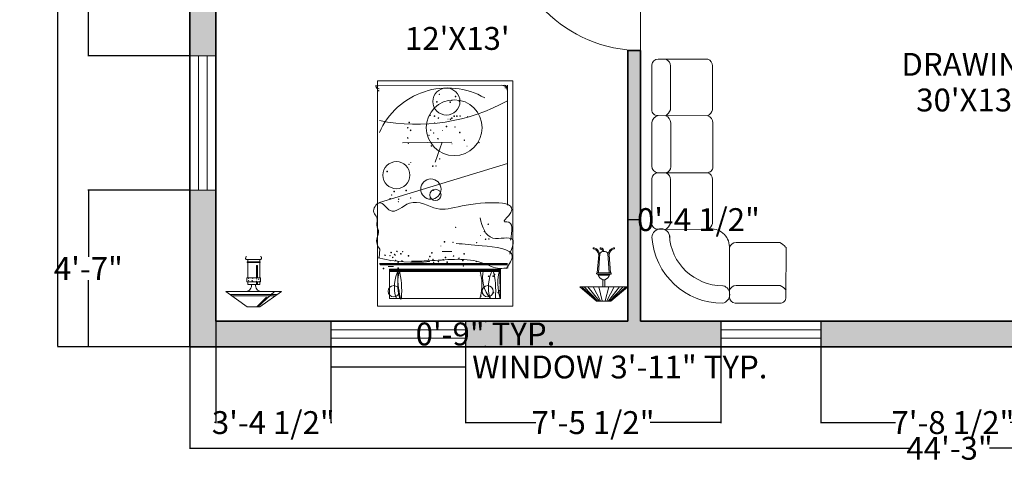
# Model space of a CAD drawing. Units: inches. Extents: x 638 to 1303, y 1 to 699.
# Tile 1 of 21: x 638 to 982, y 1 to 156. Entities that reach past the tile are written whole.
import ezdxf

# ---------------------------------------------------------------- set-up
doc = ezdxf.new("R2010")
doc.units = ezdxf.units.IN
doc.header["$MEASUREMENT"] = 0
for name, color, linetype, lineweight in [('A-ANNO-DIMS', 2, 'Continuous', 18), ('A-AREA-IDEN', 7, 'Continuous', 18), ('A-DOOR', 4, 'Continuous', 18), ('A-FURN-ACCS', 8, 'Continuous', 13), ('A-GLAZ', 4, 'Continuous', 18), ('A-WALL', 7, 'Continuous', 35), ('Furniture', 7, 'Continuous', 15)]:
    doc.layers.add(name, color=color, linetype=linetype, lineweight=lineweight)
doc.layers.add('A-WALL-PATT', color=143, linetype='Continuous', lineweight=13, true_color=0x7aafdf)
doc.styles.get("Standard").update_dxf_attribs({"font": 'arial.ttf'})
doc.dimstyles.get("Standard").update_dxf_attribs({"dimtxt": 8, "dimasz": 0.18, "dimexe": 0.18, "dimexo": 0.0625, "dimgap": 0.09, "dimtad": 0, "dimtih": 1, "dimtoh": 1, "dimdec": 4, "dimzin": 0, "dimdsep": 46, "dimlunit": 3, "dimtxsty": 'Standard', "dimcen": 0.09, "dimadec": 0, "dimazin": 0, "dimtfac": 1, "dimtdec": 4, "dimtofl": 0, "dimtmove": 0, "dimatfit": 3, "dimfxl": 1, "dimtolj": 1, "dimtzin": 0, "dimarcsym": 0})

# ---------------------------------------------------------------- blocks, each defined once
blk = doc.blocks.new('*D1')
at = {"layer": 'A-ANNO-DIMS', "color": 0, "lineweight": -2, "transparency": 16777216}
for p, q in [((697.18, 629.82), (650.92, 629.82)), ((651.1, 629.64), (651.1, 339.99)), ((651.1, 42), (651.1, 331.64)), ((697.18, 41.82), (650.92, 41.82))]:
    blk.add_line(p, q, dxfattribs=at)
at = {"layer": 'A-ANNO-DIMS', "color": 0, "transparency": 16777216}
for points in [[(651.07, 629.64), (651.13, 629.64), (651.1, 629.82)], [(651.07, 42), (651.13, 42), (651.1, 41.82)]]:
    blk.add_solid(points, dxfattribs=at)
at = {"layer": 'Defpoints', "color": 0, "transparency": 16777216}
for p in [(697.24, 629.82), (651.1, 41.82), (697.24, 41.82)]:
    blk.add_point(p, dxfattribs=at)
at = {"layer": 'A-ANNO-DIMS', "color": 0, "transparency": 16777216, "insert": (651.1, 335.82), "char_height": 8, "attachment_point": 5}
blk.add_mtext("\\A1;49'", dxfattribs=at)
blk = doc.blocks.new('DOOR-SWING-47')
for p, q in [((45, 0), (45, 46.96)), ((47, 0), (47, 47)), ((0, 0), (47, 0))]:
    blk.add_line(p, q)
blk.add_arc((47, 0), 47, 90, 180)
blk = doc.blocks.new('WIN-47')
for p, q in [((47, 9), (0, 9)), ((0, 9), (0, 0)), ((47, 0), (47, 9)), ((0, 6), (47, 6)), ((0, 3), (47, 3)), ((0, 0), (47, 0))]:
    blk.add_line(p, q)
blk = doc.blocks.new('WIN-35')
for p, q in [((35, 9), (0, 9)), ((0, 9), (0, 0)), ((35, 0), (35, 9)), ((0, 6), (35, 6)), ((0, 3), (35, 3)), ((0, 0), (35, 0))]:
    blk.add_line(p, q)
blk = doc.blocks.new('*D20')
at = {"layer": 'A-ANNO-DIMS', "color": 0, "lineweight": -2, "transparency": 16777216}
for p, q in [((746.5, 41.76), (746.5, 34.59)), ((793.5, 41.76), (793.5, 34.59)), ((746.68, 34.77), (793.32, 34.77)), ((793.5, 34.77), (793.68, 34.77))]:
    blk.add_line(p, q, dxfattribs=at)
at = {"layer": 'A-ANNO-DIMS', "color": 0, "transparency": 16777216}
for points in [[(746.68, 34.8), (746.68, 34.74), (746.5, 34.77)], [(793.32, 34.8), (793.32, 34.74), (793.5, 34.77)]]:
    blk.add_solid(points, dxfattribs=at)
at = {"layer": 'Defpoints', "color": 0, "transparency": 16777216}
for p in [(746.5, 41.82), (793.5, 41.82), (793.5, 34.77)]:
    blk.add_point(p, dxfattribs=at)
at = {"layer": 'A-ANNO-DIMS', "color": 0, "transparency": 16777216, "insert": (847.49, 34.77), "char_height": 8, "attachment_point": 5}
blk.add_mtext('\\A1;WINDOW 3\'-11" TYP.', dxfattribs=at)
blk = doc.blocks.new('*D21')
at = {"layer": 'A-ANNO-DIMS', "color": 0, "lineweight": -2, "transparency": 16777216}
for p, q in [((793.56, 50.82), (800.73, 50.82)), ((800.55, 50.64), (800.55, 50.49)), ((793.56, 41.82), (800.73, 41.82)), ((800.55, 42), (800.55, 42.14))]:
    blk.add_line(p, q, dxfattribs=at)
at = {"layer": 'A-ANNO-DIMS', "color": 0, "transparency": 16777216}
for points in [[(800.52, 50.64), (800.58, 50.64), (800.55, 50.82)], [(800.52, 42), (800.58, 42), (800.55, 41.82)]]:
    blk.add_solid(points, dxfattribs=at)
at = {"layer": 'Defpoints', "color": 0, "transparency": 16777216}
for p in [(793.5, 50.82), (800.55, 50.82), (793.5, 41.82)]:
    blk.add_point(p, dxfattribs=at)
at = {"layer": 'A-ANNO-DIMS', "color": 0, "transparency": 16777216, "insert": (800.55, 46.32), "char_height": 8, "attachment_point": 5}
blk.add_mtext('\\A1;0\'-9" TYP.', dxfattribs=at)
blk = doc.blocks.new('*D42')
at = {"layer": 'A-ANNO-DIMS', "color": 0, "lineweight": -2, "transparency": 16777216}
for p, q in [((706.237979, 50.756447), (706.237979, 15.138947)), ((746.497549, 50.756447), (746.497549, 15.138947)), ((706.057979, 15.318947), (705.877979, 15.318947)), ((746.677549, 15.318947), (746.857549, 15.318947))]:
    blk.add_line(p, q, dxfattribs=at)
at = {"layer": 'A-ANNO-DIMS', "color": 0, "transparency": 16777216}
for points in [[(706.057979, 15.348947), (706.057979, 15.288947), (706.237979, 15.318947)], [(746.677549, 15.348947), (746.677549, 15.288947), (746.497549, 15.318947)]]:
    blk.add_solid(points, dxfattribs=at)
at = {"layer": 'Defpoints', "color": 0, "transparency": 16777216}
for p in [(706.237979, 50.818947), (746.497549, 50.818947), (706.237979, 15.318947)]:
    blk.add_point(p, dxfattribs=at)
at = {"layer": 'A-ANNO-DIMS', "color": 0, "transparency": 16777216, "insert": (726.367764, 15.318947), "char_height": 8, "attachment_point": 5}
blk.add_mtext('\\A1;3\'-4 1/2"', dxfattribs=at)
blk = doc.blocks.new('*D43')
at = {"layer": 'A-ANNO-DIMS', "color": 0, "lineweight": -2, "transparency": 16777216}
for p, q in [((793.5, 50.76), (793.5, 15.14)), ((882.77, 50.76), (882.77, 15.14)), ((793.68, 15.32), (818.13, 15.32)), ((882.59, 15.32), (858.15, 15.32))]:
    blk.add_line(p, q, dxfattribs=at)
at = {"layer": 'A-ANNO-DIMS', "color": 0, "transparency": 16777216}
for points in [[(793.68, 15.35), (793.68, 15.29), (793.5, 15.32)], [(882.59, 15.35), (882.59, 15.29), (882.77, 15.32)]]:
    blk.add_solid(points, dxfattribs=at)
at = {"layer": 'Defpoints', "color": 0, "transparency": 16777216}
for p in [(793.5, 50.82), (882.77, 50.82), (793.5, 15.32)]:
    blk.add_point(p, dxfattribs=at)
at = {"layer": 'A-ANNO-DIMS', "color": 0, "transparency": 16777216, "insert": (838.14, 15.32), "char_height": 8, "attachment_point": 5}
blk.add_mtext('\\A1;7\'-5 1/2"', dxfattribs=at)
blk = doc.blocks.new('*D44')
at = {"layer": 'A-ANNO-DIMS', "color": 0, "lineweight": -2, "transparency": 16777216}
for p, q in [((917.77, 50.76), (917.77, 15.14)), ((1010.03, 50.76), (1010.03, 15.14)), ((917.95, 15.32), (943.89, 15.32)), ((1009.85, 15.32), (983.91, 15.32))]:
    blk.add_line(p, q, dxfattribs=at)
at = {"layer": 'A-ANNO-DIMS', "color": 0, "transparency": 16777216}
for points in [[(917.95, 15.35), (917.95, 15.29), (917.77, 15.32)], [(1009.85, 15.35), (1009.85, 15.29), (1010.03, 15.32)]]:
    blk.add_solid(points, dxfattribs=at)
at = {"layer": 'Defpoints', "color": 0, "transparency": 16777216}
for p in [(917.77, 50.82), (1010.03, 50.82), (917.77, 15.32)]:
    blk.add_point(p, dxfattribs=at)
at = {"layer": 'A-ANNO-DIMS', "color": 0, "transparency": 16777216, "insert": (963.9, 15.32), "char_height": 8, "attachment_point": 5}
blk.add_mtext('\\A1;7\'-8 1/2"', dxfattribs=at)
blk = doc.blocks.new('*D55')
at = {"layer": 'A-ANNO-DIMS', "color": 0, "lineweight": -2, "transparency": 16777216}
for p, q in [((697.175479, 96.574159), (661.557979, 96.574159)), ((661.737979, 96.394159), (661.737979, 73.286553)), ((661.737979, 41.998947), (661.737979, 65.106553)), ((697.175479, 41.818947), (661.557979, 41.818947))]:
    blk.add_line(p, q, dxfattribs=at)
at = {"layer": 'A-ANNO-DIMS', "color": 0, "transparency": 16777216}
for points in [[(661.707979, 96.394159), (661.767979, 96.394159), (661.737979, 96.574159)], [(661.707979, 41.998947), (661.767979, 41.998947), (661.737979, 41.818947)]]:
    blk.add_solid(points, dxfattribs=at)
at = {"layer": 'Defpoints', "color": 0, "transparency": 16777216}
for p in [(661.737979, 96.574159), (697.237979, 96.574159), (697.237979, 41.818947)]:
    blk.add_point(p, dxfattribs=at)
at = {"layer": 'A-ANNO-DIMS', "color": 0, "transparency": 16777216, "insert": (661.737979, 69.196553), "char_height": 8, "attachment_point": 5}
blk.add_mtext('\\A1;4\'-7"', dxfattribs=at)
blk = doc.blocks.new('*D56')
at = {"layer": 'A-ANNO-DIMS', "color": 0, "lineweight": -2, "transparency": 16777216}
for p, q in [((697.18, 251.22), (661.56, 251.22)), ((661.74, 251.04), (661.74, 201.62)), ((661.74, 143.75), (661.74, 193.17)), ((697.18, 143.57), (661.56, 143.57))]:
    blk.add_line(p, q, dxfattribs=at)
at = {"layer": 'A-ANNO-DIMS', "color": 0, "transparency": 16777216}
for points in [[(661.71, 251.04), (661.77, 251.04), (661.74, 251.22)], [(661.71, 143.75), (661.77, 143.75), (661.74, 143.57)]]:
    blk.add_solid(points, dxfattribs=at)
at = {"layer": 'Defpoints', "color": 0, "transparency": 16777216}
for p in [(661.74, 251.22), (697.24, 251.22), (697.24, 143.57)]:
    blk.add_point(p, dxfattribs=at)
at = {"layer": 'A-ANNO-DIMS', "color": 0, "transparency": 16777216, "insert": (661.74, 197.4), "char_height": 8, "attachment_point": 5}
blk.add_mtext('\\A1;8\'-11 1/2"', dxfattribs=at)
blk = doc.blocks.new('*D62')
at = {"layer": 'A-ANNO-DIMS', "color": 0, "lineweight": -2, "transparency": 16777216}
for p, q in [((850.24, 50.88), (850.24, 86.5)), ((850.42, 86.32), (854.56, 86.32)), ((854.74, 50.88), (854.74, 86.5)), ((854.74, 86.32), (854.92, 86.32))]:
    blk.add_line(p, q, dxfattribs=at)
at = {"layer": 'A-ANNO-DIMS', "color": 0, "transparency": 16777216}
for points in [[(850.42, 86.35), (850.42, 86.29), (850.24, 86.32)], [(854.56, 86.35), (854.56, 86.29), (854.74, 86.32)]]:
    blk.add_solid(points, dxfattribs=at)
at = {"layer": 'Defpoints', "color": 0, "transparency": 16777216}
for p in [(854.74, 86.32), (850.24, 50.82), (854.74, 50.82)]:
    blk.add_point(p, dxfattribs=at)
at = {"layer": 'A-ANNO-DIMS', "color": 0, "transparency": 16777216, "insert": (874.96, 86.32), "char_height": 8, "attachment_point": 5}
blk.add_mtext('\\A1;0\'-4 1/2"', dxfattribs=at)
blk = doc.blocks.new('*D72')
at = {"layer": 'A-ANNO-DIMS', "color": 0, "lineweight": -2, "transparency": 16777216}
for p, q in [((697.24, 41.76), (697.24, 6.14)), ((1228.24, 41.76), (1228.24, 6.14)), ((697.42, 6.32), (948.75, 6.32)), ((1228.06, 6.32), (976.73, 6.32))]:
    blk.add_line(p, q, dxfattribs=at)
at = {"layer": 'A-ANNO-DIMS', "color": 0, "transparency": 16777216}
for points in [[(697.42, 6.35), (697.42, 6.29), (697.24, 6.32)], [(1228.06, 6.35), (1228.06, 6.29), (1228.24, 6.32)]]:
    blk.add_solid(points, dxfattribs=at)
at = {"layer": 'Defpoints', "color": 0, "transparency": 16777216}
for p in [(697.24, 41.82), (1228.24, 41.82), (1228.24, 6.32)]:
    blk.add_point(p, dxfattribs=at)
at = {"layer": 'A-ANNO-DIMS', "color": 0, "transparency": 16777216, "insert": (962.74, 6.32), "char_height": 8, "attachment_point": 5}
blk.add_mtext('\\A1;44\'-3"', dxfattribs=at)

msp = doc.modelspace()

# ---------------------------------------------------------------- hatches: boundary and pattern name
at = {"layer": 'A-WALL-PATT'}
h = msp.add_hatch(color=256, dxfattribs=at)
h.dxf.hatch_style = 1
h.paths.add_polyline_path([(973.34524, 629.81895), (793.35541, 629.81895), (793.35541, 620.81895), (850.23798, 620.81895), (922.23798, 620.81895), (922.23798, 524.81895), (908.94335, 524.81895), (908.94335, 520.31895), (926.73798, 520.31895), (926.73798, 544.31895), (979.3571, 544.31895), (979.3571, 548.81895), (926.73798, 548.81895), (926.73798, 620.81895), (973.34524, 620.81895)])
h.paths.add_polyline_path([(758.35541, 629.81895), (697.23798, 629.81895), (697.23798, 586.77451), (706.23798, 586.77451), (706.23798, 620.81895), (758.35541, 620.81895)])
h.paths.add_polyline_path([(1075.85281, 629.81895), (1003.34524, 629.81895), (1003.34524, 620.81895), (1046.73798, 620.81895), (1046.73798, 560.81895), (1046.73798, 548.81895), (1026.3571, 548.81895), (1026.3571, 544.31895), (1046.73798, 544.31895), (1046.73798, 486.87457), (1051.23798, 486.87457), (1051.23798, 556.31895), (1162.89753, 556.31895), (1162.89753, 560.81895), (1051.23798, 560.81895), (1051.23798, 620.81895), (1075.85281, 620.81895)])
h.paths.add_polyline_path([(1228.23798, 629.81895), (1105.85281, 629.81895), (1105.85281, 620.81895), (1219.23798, 620.81895), (1219.23798, 560.81895), (1197.89753, 560.81895), (1197.89753, 556.31895), (1219.23798, 556.31895), (1219.23798, 498.80084), (1228.23798, 498.80084)])
h.paths.add_polyline_path([(1051.23798, 439.87457), (1046.73798, 439.87457), (1046.73798, 407.81895), (1219.23798, 407.81895), (1219.23798, 381.66175), (1228.23798, 381.66175), (1228.23798, 451.80084), (1219.23798, 451.80084), (1219.23798, 412.31895), (1051.23798, 412.31895)])
h.paths.add_polyline_path([(1228.23798, 346.66175), (1219.23798, 346.66175), (1219.23798, 335.81895), (1046.73798, 335.81895), (1046.73798, 273.56895), (1051.23798, 273.56895), (1051.23798, 331.31895), (1219.23798, 331.31895), (1219.23798, 308.99654), (1228.23798, 308.99654)])
h.paths.add_polyline_path([(1228.23798, 261.99654), (1219.23798, 261.99654), (1219.23798, 211.31895), (1051.23798, 211.31895), (1051.23798, 226.56895), (1046.73798, 226.56895), (1046.73798, 211.31895), (983.84714, 211.31895), (983.84714, 206.81895), (1219.23798, 206.81895), (1219.23798, 166.83987), (1228.23798, 166.83987)])
h.paths.add_polyline_path([(1228.23798, 119.83987), (1219.23798, 119.83987), (1219.23798, 50.81895), (1197.89277, 50.81895), (1197.89277, 41.81895), (1228.23798, 41.81895)])
h.paths.add_polyline_path([(1162.89277, 50.81895), (1069.02949, 50.81895), (1069.02949, 41.81895), (1162.89277, 41.81895)])
h.paths.add_polyline_path([(1010.02949, 50.81895), (941.89631, 50.81895), (917.77455, 50.81895), (917.77455, 41.81895), (941.89631, 41.81895), (1010.02949, 41.81895)])
h.paths.add_polyline_path([(882.77455, 50.81895), (854.73798, 50.81895), (854.73798, 145.50379), (850.23798, 145.50379), (850.23798, 50.81895), (793.49755, 50.81895), (793.49755, 41.81895), (882.77455, 41.81895)])
h.paths.add_polyline_path([(746.49755, 50.81895), (706.23798, 50.81895), (706.23798, 96.57416), (697.23798, 96.57416), (697.23798, 41.81895), (746.49755, 41.81895)])
h.paths.add_polyline_path([(706.23798, 206.81895), (714.01165, 206.81895), (714.01165, 211.31895), (706.23798, 211.31895), (706.23798, 251.21966), (697.23798, 251.21966), (697.23798, 143.57416), (706.23798, 143.57416)])
h.paths.add_polyline_path([(923.84714, 211.31895), (854.73798, 211.31895), (854.73798, 397.8313), (850.23798, 397.8313), (850.23798, 388.31895), (747.9539, 388.31895), (747.9539, 383.81895), (850.23798, 383.81895), (850.23798, 311.81895), (706.23798, 311.81895), (706.23798, 342.78787), (697.23798, 342.78787), (697.23798, 281.21966), (706.23798, 281.21966), (706.23798, 307.31895), (850.23798, 307.31895), (850.23798, 211.31895), (749.01165, 211.31895), (749.01165, 206.81895), (850.23798, 206.81895), (850.23798, 192.50379), (854.73798, 192.50379), (854.73798, 206.81895), (923.84714, 206.81895)])
h.paths.add_polyline_path([(706.23798, 434.70471), (697.23798, 434.70471), (697.23798, 372.78787), (706.23798, 372.78787), (706.23798, 383.81895), (712.9539, 383.81895), (712.9539, 388.31895), (706.23798, 388.31895)])
h.paths.add_polyline_path([(706.23798, 520.31895), (850.23798, 520.31895), (850.23798, 444.8313), (854.73798, 444.8313), (854.73798, 520.31895), (861.94335, 520.31895), (861.94335, 524.81895), (706.23798, 524.81895), (706.23798, 551.77451), (697.23798, 551.77451), (697.23798, 481.70471), (706.23798, 481.70471)])

# ---------------------------------------------------------------- linework, layer by layer
at = {"layer": 'A-FURN-ACCS'}
for p, q in [((721.62646, 72.31504), (717.42875, 72.31504)), ((717.42875, 72.31504), (717.42875, 65.97048)), ((721.62646, 65.97048), (721.62646, 72.31504)), ((839.60939, 67.69738), (840.09801, 73.96329)), ((840.0019, 67.66677), (840.53154, 74.45866)), ((843.81707, 67.66677), (843.28744, 74.45866)), ((844.20958, 67.69738), (843.72096, 73.96329)), ((844.20958, 67.69738), (843.72096, 73.96329)), ((721.83123, 71.59872), (717.22398, 71.59872)), ((717.22398, 71.59872), (717.22398, 71.34289)), ((717.22398, 71.34289), (721.83123, 71.34289)), ((720.55144, 70.31957), (720.55144, 65.97048)), ((720.90978, 70.31957), (720.55144, 70.31957)), ((720.90978, 65.97048), (720.90978, 70.31957)), ((721.83123, 71.34289), (721.83123, 71.59872)), ((721.88242, 65.97048), (717.17279, 65.97048)), ((717.17279, 65.97048), (717.17279, 64.58901)), ((717.73994, 65.79158), (717.70003, 65.67263)), ((717.83798, 65.72543), (717.70015, 65.67252)), ((717.83798, 65.72543), (717.74007, 65.79147)), ((719.11023, 65.86473), (719.13197, 65.67778)), ((719.28542, 65.83746), (719.11035, 65.86462)), ((719.28542, 65.83746), (719.1321, 65.67767)), ((720.56893, 65.63393), (720.52902, 65.51497)), ((720.66697, 65.56777), (720.52914, 65.51487)), ((720.66697, 65.56777), (720.56906, 65.63382)), ((721.21109, 65.5389), (721.23284, 65.35195)), ((721.38629, 65.51164), (721.21122, 65.53879)), ((721.38629, 65.51164), (721.23296, 65.35184)), ((721.88242, 64.58901), (721.88242, 65.97048)), ((840.0019, 67.66677), (839.53319, 67.66677)), ((839.9712, 67.27307), (839.53319, 67.27307)), ((839.94099, 66.88565), (839.9712, 67.27307)), ((843.87799, 66.88565), (839.94099, 66.88565)), ((843.84778, 67.27307), (839.9712, 67.27307)), ((843.81707, 67.66677), (840.0019, 67.66677)), ((844.32785, 67.66677), (843.81707, 67.66677)), ((844.32785, 67.27307), (843.84778, 67.27307)), ((843.87799, 66.88565), (843.84778, 67.27307)), ((717.17279, 64.58901), (721.88242, 64.58901)), ((717.42875, 64.58901), (717.42875, 63.61686)), ((717.42875, 63.61686), (721.62646, 63.61686)), ((717.69258, 65.06673), (717.71535, 64.94334)), ((717.81037, 65.05633), (717.69271, 65.06662)), ((717.81037, 65.05633), (717.71547, 64.94323)), ((718.91495, 64.99903), (718.87504, 64.88007)), ((719.013, 64.93287), (718.87516, 64.87996)), ((719.013, 64.93287), (718.91508, 64.99892)), ((719.10451, 64.9432), (719.12727, 64.81981)), ((719.2223, 64.9328), (719.10464, 64.94309)), ((719.2223, 64.9328), (719.1274, 64.8197)), ((720.51644, 64.81967), (720.5392, 64.69628)), ((720.63422, 64.80927), (720.51656, 64.81957)), ((720.63422, 64.80927), (720.53932, 64.69617)), ((720.55144, 64.58901), (720.55144, 63.61686)), ((720.55144, 63.61686), (720.90978, 63.61686)), ((720.90978, 63.61686), (720.90978, 64.58901)), ((721.62646, 63.61686), (721.62646, 64.58901)), ((721.74394, 64.84137), (721.70403, 64.72242)), ((721.84199, 64.77522), (721.70415, 64.72231)), ((721.84199, 64.77522), (721.74407, 64.84126)), ((833.52293, 62.81708), (839.35639, 57.82954)), ((850.23798, 62.81708), (833.52293, 62.81708)), ((834.19758, 62.81708), (839.55305, 57.83485)), ((835.05292, 62.81708), (839.83199, 57.84238)), ((836.33652, 62.81708), (840.23356, 57.85323)), ((838.20029, 62.81708), (840.75347, 57.86728)), ((840.12565, 62.81708), (841.36533, 57.8838)), ((842.30319, 65.31085), (841.51579, 65.31085)), ((841.51579, 62.81708), (841.51579, 65.31085)), ((842.30319, 62.81708), (842.30319, 65.31085)), ((843.63526, 62.81708), (842.39558, 57.8838)), ((845.56063, 62.81708), (843.00744, 57.86728)), ((847.4244, 62.81708), (843.52735, 57.85323)), ((848.70799, 62.81708), (843.92892, 57.84238)), ((849.56333, 62.81708), (844.20786, 57.83485)), ((850.23798, 62.81708), (844.40452, 57.82954)), ((729.18484, 61.22243), (709.75571, 61.22243)), ((717.26321, 55.80309), (709.75571, 61.22243)), ((727.59959, 60.09382), (711.18104, 60.09382)), ((727.07837, 59.7031), (711.76742, 59.7031)), ((720.56307, 55.7959), (723.95102, 59.24726)), ((720.95399, 55.7959), (726.7526, 61.20086)), ((721.67734, 55.80309), (729.18484, 61.22243)), ((721.67734, 55.80309), (717.26321, 55.80309)), ((844.40452, 57.82954), (839.35639, 57.82954))]:
    msp.add_line(p, q, dxfattribs=at)
for centre, radius, start, end in [((838.41821, 76.24622), 0.19985, 64.8779516, 264.742049), ((837.79541, 73.82081), 2.30701, 2.933841, 74.8100003), ((837.79541, 73.82081), 2.70071, 2.933841, 74.8100003), ((840.77094, 76.23752), 0.20201, 69.8469138, 275.801077), ((840.68791, 75.21492), 0.82811, 354.9969401, 82.8239954), ((840.68791, 75.21492), 1.22181, 358.8637261, 82.8239954), ((846.02356, 73.82081), 2.70071, 105.1899997, 177.066159), ((846.02356, 73.82081), 2.30701, 105.1899997, 177.066159), ((845.40077, 76.24622), 0.19985, 275.257951, 115.1220484), ((717.27181, 72.90823), 0.5947, 116.4475321, 274.077556), ((721.66875, 72.90823), 0.5947, 265.922444, 63.5524679), ((841.90949, 73.52777), 1.66292, 34.0415049, 145.9584951), ((839.53622, 67.46992), 0.19687, 90.8813941, 269.1186059), ((842.3421, 67.71196), 2.53931, 198.9902213, 251.0097787), ((841.47688, 67.71196), 2.53931, 288.9902213, 341.0097787), ((844.32482, 67.46992), 0.19687, 270.8813941, 89.1186059), ((716.71653, 63.26816), 2.06065, 273.807658, 9.7421638), ((722.22402, 63.26816), 2.06065, 170.2578362, 266.192342)]:
    msp.add_arc(centre, radius, start, end, dxfattribs=at)
at = {"layer": 'A-WALL'}
for p, q in [((697.23798, 41.81895), (697.23798, 629.81895)), ((706.23798, 50.81895), (706.23798, 206.81895)), ((850.23798, 50.81895), (850.23798, 145.50379)), ((850.23798, 145.50379), (854.73798, 145.50379)), ((854.73798, 50.81895), (854.73798, 145.50379)), ((850.23798, 50.81895), (706.23798, 50.81895)), ((941.89631, 50.81895), (854.73798, 50.81895)), ((1010.02949, 50.81895), (941.89631, 50.81895)), ((941.89631, 41.81895), (697.23798, 41.81895)), ((1228.23798, 41.81895), (941.89631, 41.81895))]:
    msp.add_line(p, q, dxfattribs=at)
at = {"layer": 'Furniture'}
for p, q in [((878.21123, 142.4275), (860.83446, 142.4275)), ((858.67362, 140.44573), (858.67362, 124.7717)), ((865.17128, 124.68162), (865.17128, 140.08541)), ((879.9219, 124.68162), (879.9219, 140.08541)), ((762.80981, 56.07859), (762.80981, 134.81859)), ((762.80981, 134.81859), (810.05381, 134.81859)), ((810.05381, 134.81859), (810.05381, 56.07859)), ((807.01616, 133.3263), (762.13218, 133.09941)), ((808.06723, 132.40064), (807.27983, 132.40064)), ((808.19726, 91.3241), (808.19726, 133.3344)), ((808.19726, 91.3241), (808.19726, 131.3578)), ((860.83446, 122.69985), (878.30127, 122.60977)), ((858.67362, 120.26767), (858.67362, 105.04405)), ((865.26132, 116.30413), (865.26132, 120.17759)), ((880.01194, 116.30413), (880.01194, 120.17759)), ((865.26132, 104.77381), (865.26132, 116.30413)), ((880.01194, 104.77381), (880.01194, 116.30413)), ((771.53805, 113.14485), (788.77747, 113.37175)), ((782.98374, 106.43895), (785.36337, 113.37481)), ((808.21877, 105.89322), (763.45403, 92.2881)), ((808.19257, 106.18712), (808.19257, 91.61098)), ((858.67362, 100.72395), (858.67362, 85.04993)), ((860.65439, 102.70196), (877.94113, 102.70196)), ((878.21123, 102.70572), (860.83446, 102.70572)), ((865.17128, 84.95984), (865.17128, 100.36363)), ((879.9219, 84.95984), (879.9219, 100.36363)), ((860.83446, 82.97807), (878.30127, 82.88799)), ((763.64904, 75.9642), (763.43252, 72.91644)), ((885.8105, 76.62499), (885.8105, 59.24822)), ((903.55638, 78.33565), (888.1526, 78.33565)), ((905.62824, 76.71502), (905.53816, 59.24822)), ((785.35393, 75.14265), (788.77747, 75.14265)), ((808.21877, 70.99543), (763.45403, 70.9756)), ((808.21877, 70.69685), (763.45403, 70.67702)), ((808.19726, 70.54754), (763.75292, 70.52771)), ((766.56768, 69.91577), (768.4091, 69.91577)), ((805.5645, 68.86561), (766.97341, 68.86561)), ((767.00563, 58.71898), (767.00563, 69.04444)), ((767.00563, 69.04444), (805.76692, 69.04444)), ((805.71263, 58.73116), (805.5645, 68.86561)), ((805.76692, 69.04444), (805.76692, 58.71898)), ((805.5645, 68.74205), (766.97341, 68.74205)), ((805.5645, 68.44343), (766.97341, 68.44343)), ((805.5645, 68.14489), (766.97341, 68.14489)), ((903.55638, 63.23723), (888.1526, 63.23723)), ((805.76692, 58.71898), (767.00563, 58.71898)), ((885.8105, 61.52656), (885.8105, 61.46443)), ((762.80981, 56.07859), (810.05381, 56.07859)), ((887.79228, 57.08737), (903.4663, 57.08737))]:
    msp.add_line(p, q, dxfattribs=at)
for centre, radius in [((786.8866, 127.62421), 4.7244), ((789.61602, 118.47754), 9.76451), ((783.5393, 127.47689), 0.11811), ((784.38111, 130.15834), 0.07874), ((788.22711, 127.42812), 0.11811), ((788.7936, 127.94244), 0.03937), ((790.10171, 129.36745), 0.11811), ((791.47065, 127.7687), 0.11811), ((781.17459, 122.79126), 0.11811), ((782.71002, 122.54431), 0.11811), ((784.08796, 121.85478), 0.11811), ((787.42466, 121.46399), 0.03937), ((788.27641, 121.42292), 0.11811), ((788.77576, 121.80601), 0.11811), ((789.60505, 122.49907), 0.11811), ((790.558, 122.5272), 0.11811), ((791.67514, 122.58824), 0.07874), ((794.29067, 122.2234), 0.11811), ((773.34192, 118.47162), 0.11811), ((773.90015, 120.28444), 0.11811), ((774.35644, 117.54976), 0.11811), ((781.37908, 117.6108), 0.07874), ((782.74802, 120.11762), 0.07874), ((785.59936, 117.49109), 0.03937), ((786.90747, 118.9161), 0.11811), ((789.84984, 118.74928), 0.07874), ((773.34192, 114.89498), 0.11811), ((780.82086, 115.79798), 0.07874), ((783.93305, 114.61931), 0.11811), ((791.53479, 116.77236), 0.11811), ((793.10823, 114.09872), 0.07874), ((773.53742, 113.04482), 0.07874), ((781.63088, 112.08036), 0.11811), ((788.85774, 112.84053), 0.03937), ((794.04139, 112.02169), 0.03937), ((798.29188, 113.27988), 0.07874), ((784.57325, 107.58202), 0.07874), ((769.4036, 101.86749), 4.7244), ((766.17475, 103.1427), 0.11811), ((773.81175, 105.68623), 0.07874), ((774.41727, 106.32384), 0.03937), ((782.08717, 105.01416), 0.11811), ((783.20431, 105.0752), 0.07874), ((781.45384, 96.99379), 3.5433), ((772.79327, 96.52197), 0.11811), ((783.02493, 94.94924), 1.9685), ((767.23011, 93.62399), 0.11811), ((767.74818, 94.91775), 0.07874), ((768.59905, 96.13081), 0.11811), ((770.17248, 93.45716), 0.07874), ((774.36671, 93.84833), 0.07874), ((781.2142, 93.65957), 0.03937), ((770.11622, 92.59014), 0.03937), ((790.07802, 83.61536), 0.07874), ((801.50973, 84.69376), 0.11811), ((798.83268, 80.76193), 0.03937), ((800.14079, 82.18694), 0.11811), ((800.59708, 79.45226), 0.11811), ((801.71423, 79.5133), 0.07874), ((784.91489, 77.11567), 0.03937), ((786.223, 78.54068), 0.11811), ((789.16537, 78.37385), 0.07874), ((797.46374, 78.25511), 0.03937), ((765.44288, 73.83099), 0.11811), ((767.19953, 73.72267), 0.07874), ((767.55269, 74.77378), 0.11811), ((768.10134, 73.1233), 0.11811), ((768.7093, 74.19174), 0.03937), ((768.93062, 73.95031), 0.11811), ((769.57985, 75.2058), 0.11811), ((770.95779, 74.38233), 0.11811), ((771.60767, 75.07924), 0.07874), ((773.61625, 73.67464), 0.11811), ((780.66554, 72.46448), 0.03937), ((781.13221, 73.39897), 0.11811), ((781.78144, 74.65446), 0.11811), ((782.157, 72.37581), 0.07874), ((785.7424, 72.24751), 0.11811), ((786.57169, 73.07452), 0.11811), ((789.37455, 73.59358), 0.07874), ((791.25731, 72.79885), 0.11811), ((793.03539, 74.34107), 0.11811), ((764.89423, 69.2014), 0.11811), ((767.34036, 71.68492), 0.03937), ((768.58661, 70.73369), 0.03937), ((769.12612, 72.10014), 0.07874), ((770.01741, 69.33667), 0.11811), ((770.03424, 71.47281), 0.11811), ((771.38635, 71.8435), 0.11811), ((773.30327, 70.5943), 0.11811), ((784.06201, 71.63668), 0.11811), ((787.12034, 71.42404), 0.11811), ((792.63525, 71.97537), 0.11811), ((792.83075, 70.12521), 0.07874), ((797.32088, 71.6997), 0.11811), ((798.32165, 66.66202), 0.03937), ((801.62618, 66.50475), 0.11811), ((803.20593, 66.50475), 0.11811), ((803.67575, 67.13384), 0.11811), ((768.45628, 61.27379), 1.9685), ((801.30448, 61.25507), 1.9685), ((799.09726, 60.62774), 0.03937), ((799.09726, 59.52506), 0.03937), ((800.677, 59.52506), 0.03937), ((801.14682, 60.15416), 0.03937), ((803.34774, 60.78325), 0.07874), ((804.92749, 60.78325), 0.07874), ((805.39731, 61.41234), 0.07874)]:
    msp.add_circle(centre, radius, dxfattribs=at)
for centre, radius, start, end in [((860.83446, 140.25857), 2.16893, 90, 175.0497532), ((862.71265, 140.08541), 2.45863, 0, 64.0743186), ((877.46327, 140.08541), 2.45863, 0, 72.2887697), ((763.25047, 133.23733), 1.12676, 187.0311135, 279.2977379), ((763.59987, 132.34211), 1.01799, 131.933732, 260.5377885), ((787.31456, 106.28258), 26.07963, 60.150566, 156.1930898), ((806.22876, 131.3578), 1.9685, 0, 90), ((807.01616, 132.1452), 1.1811, 0, 90), ((776.3701, 185.18732), 65.53325, 258.6330491, 299.0775249), ((860.74731, 124.7717), 2.07369, 180, 272.4088158), ((860.51717, 126.65236), 5.05416, 306.8838019, 337.0502276), ((875.26779, 126.65236), 5.05416, 306.8838019, 337.0502276), ((861.69169, 119.76228), 3.06009, 106.2679921, 170.493691), ((862.67698, 120.17759), 2.58433, 0, 70.2411232), ((877.4276, 120.17759), 2.58433, 0, 70.2411232), ((861.04867, 105.04405), 2.37505, 180, 260.4441563), ((863.19051, 104.77276), 2.07081, 286.7577384, 0.0289611), ((877.94113, 104.77276), 2.07081, 270, 0.0289611), ((860.83446, 100.53679), 2.16893, 90, 175.0497532), ((862.71265, 100.36363), 2.45863, 0, 64.0743186), ((877.46327, 100.36363), 2.45863, 0, 72.2887697), ((860.74731, 85.04993), 2.07369, 180, 272.4088158), ((861.84125, 80.00583), 3.14085, 358.012128, 178.012128), ((860.51717, 86.93058), 5.05416, 306.8838019, 337.0502276), ((875.26779, 86.93058), 5.05416, 306.8838019, 337.0502276), ((879.55291, 76.85253), 6.21314, 0, 100.6006241), ((883.43485, 81.85147), 24.79222, 183.9870353, 269.9482795), ((883.43485, 81.85147), 18.64508, 182.9159372, 270), ((888.1526, 75.87702), 2.45863, 90, 162.2887697), ((901.40468, 73.62287), 5.05416, 36.8838019, 67.0502276), ((775.8361, 123.85369), 52.4617, 255.8436923, 275.7821453), ((780.69639, 62.84349), 12.01174, 149.807163, 199.9256392), ((787.3481, 63.78727), 17.50229, 163.1328927, 196.7592723), ((742.43113, 61.57536), 28.82509, 354.7073772, 14.688459), ((781.42789, 63.75122), 17.84721, 343.663399, 17.1742517), ((810.913, 66.08592), 11.36252, 165.8396069, 220.3370289), ((813.54459, 62.82476), 12.01174, 149.807163, 199.9256392), ((775.27934, 61.55663), 28.82509, 354.7073772, 14.688459), ((821.36835, 64.03231), 16.5259, 163.0006196, 198.6759461), ((800.74757, 66.28082), 30.84648, 175.6160505, 194.8863201), ((882.72855, 60.16316), 3.17835, 282.426075, 73.2334882), ((888.1526, 60.7786), 2.45863, 90, 162.2887697), ((901.58564, 58.58312), 5.05416, 36.8838019, 67.0502276), ((887.97944, 59.24822), 2.16893, 180, 265.0497532), ((903.4663, 59.16106), 2.07369, 270, 2.4088158)]:
    msp.add_arc(centre, radius, start, end, dxfattribs=at)
for points, knots in [([(809.2814, 79.08492), (809.83927, 82.31299), (810.46709, 85.94581), (806.17596, 85.36276), (815.88654, 93.85292), (792.53352, 91.90724), (783.76921, 88.68452), (774.69707, 95.00147), (767.74308, 86.63159), (763.75951, 94.25376), (760.53095, 89.08537), (763.19007, 87.04326), (762.13118, 84.3453), (763.75619, 81.74839), (761.81595, 78.83241), (763.02866, 76.9349), (763.64904, 75.9642)], [0, 0, 0, 0, 6.608380599, 7.436977867, 10.160478595, 26.828110157, 35.651645641, 45.441606877, 52.697614321, 57.347481326, 61.162366278, 63.231685286, 65.951855508, 68.505046126, 71.545851705, 74.730692399, 74.730692399, 74.730692399, 74.730692399]), ([(809.01571, 74.25809), (809.86144, 76.41657), (811.81636, 81.40596), (801.00489, 77.91528), (799.47106, 83.76646), (798.62788, 86.98297)], [0, 0, 0, 0, 5.247260809, 12.129134869, 20.530793364, 20.530793364, 20.530793364, 20.530793364]), ([(807.85369, 69.24274), (808.87789, 70.79354), (812.32651, 76.0153), (798.99496, 77.18731), (793.00933, 77.74489), (790.32872, 77.99459)], [0, 0, 0, 0, 4.712341894, 15.867179444, 24.914550184, 24.914550184, 24.914550184, 24.914550184]), ([(774.68828, 71.73602), (777.05169, 71.78335), (785.31866, 71.94891), (796.06716, 73.45365), (804.3829, 68.86761), (807.46397, 69.32959), (808.46224, 69.47927)], [0, 0, 0, 0, 7.121262186, 24.909491295, 31.123221053, 34.101393508, 34.101393508, 34.101393508, 34.101393508])]:
    msp.add_open_spline(points, degree=3, knots=knots, dxfattribs=at)
for p in [(782.47673, 116.65264), (782.47673, 96.57312), (782.47673, 71.35719)]:
    msp.add_point(p, dxfattribs=at)

# ---------------------------------------------------------------- block references
at = {"layer": 'A-DOOR', "rotation": 90.00000000000033}
msp.add_blockref('DOOR-SWING-47', (854.73793, 145.50344), dxfattribs=at)
at = {"layer": 'A-GLAZ', "rotation": 270}
msp.add_blockref('WIN-47', (697.23803, 143.57371), dxfattribs=at)
at = {"layer": 'A-GLAZ'}
for name, p in [('WIN-47', (746.498, 41.819)), ('WIN-35', (882.77478, 41.819))]:
    msp.add_blockref(name, p, dxfattribs=at)

# ---------------------------------------------------------------- texts
at = {"layer": 'A-AREA-IDEN'}
for s, p in [("12'X13'", (772.41, 145.69683)), ('DRAWING ROOM', (945.90204, 136.63087)), ("30'X13'", (951.07931, 124.1548))]:
    msp.add_text(s, height=8, dxfattribs=at).set_placement(p)

# ---------------------------------------------------------------- dimensions: what is measured, and where the dimension line sits
at = {"layer": 'A-ANNO-DIMS'}
for base, p1, p2, angle, override, picture, middle in [((651.10111, 41.81895), (697.23798, 629.81895), (697.23798, 41.81895), 90, {"dimclrd": 0, "dimclre": 0, "dimclrt": 0}, '*D1', (651.10111, 335.81895)), ((661.73798, 251.21966), (697.23798, 143.57416), (697.23798, 251.21966), 90, {"dimdec": 1, "dimlfac": 1, "dimrnd": 0, "dimzin": 1, "dimdsep": 46, "dimlunit": 4, "dimfrac": 2}, '*D56', (661.73798, 197.39691)), ((661.73798, 96.57416), (697.23798, 41.81895), (697.23798, 96.57416), 90, {"dimdec": 1, "dimlfac": 1, "dimrnd": 0, "dimzin": 1, "dimdsep": 46, "dimlunit": 4, "dimfrac": 2}, '*D55', (661.73798, 69.19655)), ((854.73798, 86.31895), (850.23798, 50.81895), (854.73798, 50.81895), 0, {"dimdec": 1, "dimlfac": 1, "dimrnd": 0, "dimzin": 1, "dimdsep": 46, "dimlunit": 4, "dimfrac": 2}, '*D62', (874.96159, 86.31895)), ((706.23798, 15.31895), (746.49755, 50.81895), (706.23798, 50.81895), 180, {"dimdec": 1, "dimlfac": 1, "dimrnd": 0, "dimzin": 1, "dimdsep": 46, "dimlunit": 4, "dimfrac": 2}, '*D42', (726.36776, 15.31895)), ((793.49755, 15.31895), (882.77455, 50.81895), (793.49755, 50.81895), 180, {"dimdec": 1, "dimlfac": 1, "dimrnd": 0, "dimzin": 1, "dimdsep": 46, "dimlunit": 4, "dimfrac": 2}, '*D43', (838.13605, 15.31895)), ((917.77455, 15.31895), (1010.02949, 50.81895), (917.77455, 50.81895), 180, {"dimdec": 1, "dimlfac": 1, "dimrnd": 0, "dimzin": 1, "dimdsep": 46, "dimlunit": 4, "dimfrac": 2}, '*D44', (963.90202, 15.31895))]:
    dim = msp.add_linear_dim(base=base, p1=p1, p2=p2, angle=angle, dimstyle='Standard', override=override, dxfattribs=at)
    dim.commit()
    dim.dimension.update_dxf_attribs({"geometry": picture, "text_midpoint": middle})
dim = msp.add_linear_dim(base=(800.54755, 50.81895), p1=(793.49755, 41.81895), p2=(793.49755, 50.81895), angle=90, text='<> TYP.', dimstyle='Standard', override={"dimdec": 1, "dimlfac": 1, "dimrnd": 0, "dimzin": 1, "dimdsep": 46, "dimlunit": 4, "dimfrac": 2}, dxfattribs=at)
dim.commit()
dim.dimension.update_dxf_attribs({"geometry": '*D21', "text_midpoint": (800.54755, 46.31895)})
dim = msp.add_linear_dim(base=(793.49755, 34.76895), p1=(746.49755, 41.81895), p2=(793.49755, 41.81895), text='WINDOW <> TYP.', dimstyle='Standard', override={"dimdec": 1, "dimlfac": 1, "dimrnd": 0, "dimzin": 1, "dimdsep": 46, "dimlunit": 4, "dimfrac": 2}, dxfattribs=at)
dim.commit()
dim.dimension.update_dxf_attribs({"geometry": '*D20', "text_midpoint": (847.49197, 34.76895)})
dim = msp.add_linear_dim(base=(1228.23798, 6.31895), p1=(697.23798, 41.81895), p2=(1228.23798, 41.81895), dimstyle='Standard', override={"dimdec": 1, "dimlfac": 1, "dimrnd": 0, "dimzin": 1, "dimdsep": 46, "dimlunit": 4, "dimfrac": 2}, dxfattribs=at)
dim.commit()
dim.dimension.update_dxf_attribs({"geometry": '*D72', "text_midpoint": (962.73798, 6.31895)})

doc.saveas('drawing.dxf')
